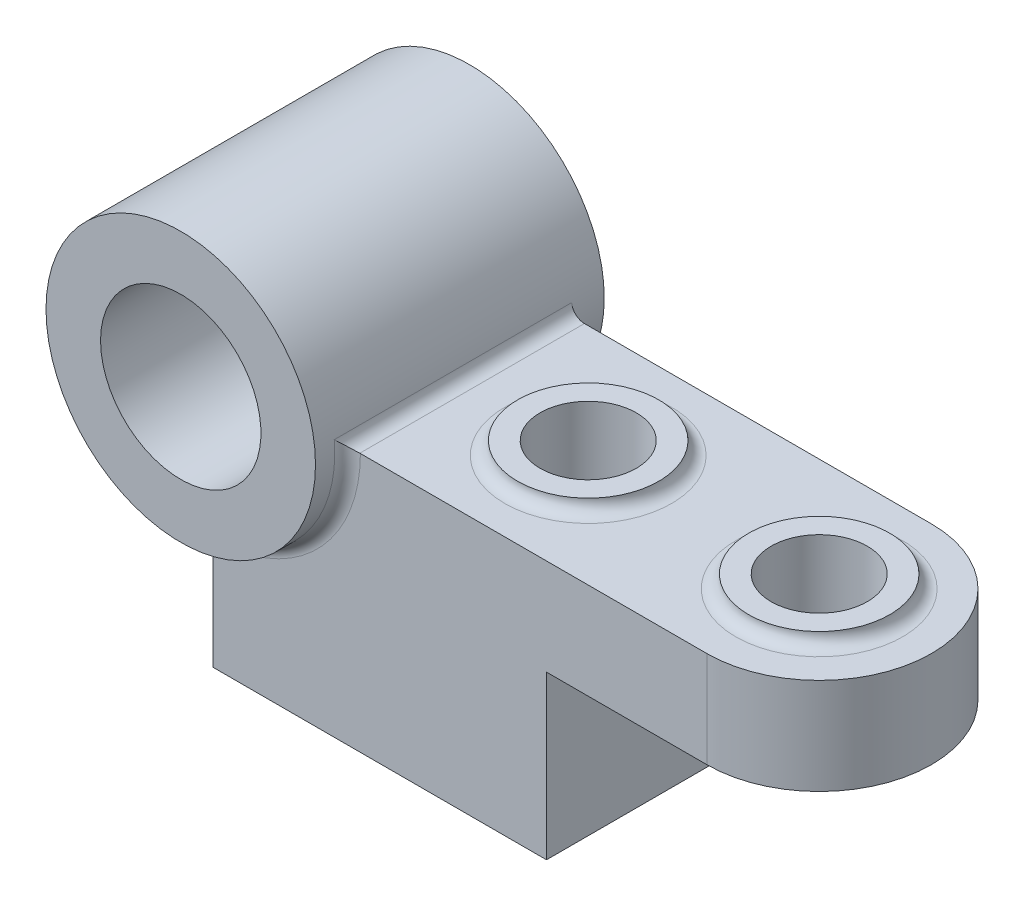
ISO-10303-21;
HEADER;
FILE_DESCRIPTION(('STEP AP214'),'2;1');
FILE_NAME('part.step','',(''),(''),'','','');
FILE_SCHEMA(('AUTOMOTIVE_DESIGN { 1 0 10303 214 1 1 1 1 }'));
ENDSEC;
DATA;
#1=APPLICATION_CONTEXT('core data for automotive mechanical design processes');
#2=APPLICATION_PROTOCOL_DEFINITION('international standard','automotive_design',2000,#1);
#3=PRODUCT_CONTEXT('',#1,'mechanical');
#4=PRODUCT('Part','Part','',(#3));
#5=PRODUCT_RELATED_PRODUCT_CATEGORY('part','',(#4));
#6=PRODUCT_DEFINITION_FORMATION('','',#4);
#7=PRODUCT_DEFINITION_CONTEXT('part definition',#1,'design');
#8=PRODUCT_DEFINITION('design','',#6,#7);
#9=PRODUCT_DEFINITION_SHAPE('','',#8);
#10=(LENGTH_UNIT() NAMED_UNIT(*) SI_UNIT(.MILLI.,.METRE.));
#11=(NAMED_UNIT(*) PLANE_ANGLE_UNIT() SI_UNIT($,.RADIAN.));
#12=(NAMED_UNIT(*) SI_UNIT($,.STERADIAN.) SOLID_ANGLE_UNIT());
#13=UNCERTAINTY_MEASURE_WITH_UNIT(LENGTH_MEASURE(1.E-05),#10,'distance_accuracy_value','');
#14=(GEOMETRIC_REPRESENTATION_CONTEXT(3) GLOBAL_UNCERTAINTY_ASSIGNED_CONTEXT((#13)) GLOBAL_UNIT_ASSIGNED_CONTEXT((#10,
#11,#12)) REPRESENTATION_CONTEXT('',''));
#15=CARTESIAN_POINT('',(0.,0.,0.));
#16=DIRECTION('',(0.,0.,1.));
#17=DIRECTION('',(1.,0.,0.));
#18=AXIS2_PLACEMENT_3D('',#15,#16,#17);
#19=CARTESIAN_POINT('',(0.,-15.,17.5));
#20=DIRECTION('',(0.,-1.,0.));
#21=DIRECTION('',(0.,0.,-1.));
#22=AXIS2_PLACEMENT_3D('',#19,#20,#21);
#23=PLANE('',#22);
#24=CARTESIAN_POINT('',(77.,-15.,0.));
#25=DIRECTION('',(0.,-1.,0.));
#26=DIRECTION('',(0.,0.,-1.));
#27=AXIS2_PLACEMENT_3D('',#24,#25,#26);
#28=CIRCLE('',#27,17.5);
#29=CARTESIAN_POINT('',(77.,-15.,17.5));
#30=VERTEX_POINT('',#29);
#31=CARTESIAN_POINT('',(77.,-15.,-17.5));
#32=VERTEX_POINT('',#31);
#33=EDGE_CURVE('E153',#30,#32,#28,.F.);
#34=ORIENTED_EDGE('',*,*,#33,.F.);
#35=DIRECTION('',(-1.,0.,0.));
#36=VECTOR('',#35,1.);
#37=CARTESIAN_POINT('',(0.,-15.,17.5));
#38=LINE('',#37,#36);
#39=CARTESIAN_POINT('',(52.,-15.,17.5));
#40=VERTEX_POINT('',#39);
#41=EDGE_CURVE('E180',#30,#40,#38,.T.);
#42=ORIENTED_EDGE('',*,*,#41,.T.);
#43=DIRECTION('',(0.,0.,-1.));
#44=VECTOR('',#43,1.);
#45=CARTESIAN_POINT('',(52.,-15.,17.5));
#46=LINE('',#45,#44);
#47=CARTESIAN_POINT('',(52.,-15.,-17.5));
#48=VERTEX_POINT('',#47);
#49=EDGE_CURVE('E182',#40,#48,#46,.T.);
#50=ORIENTED_EDGE('',*,*,#49,.T.);
#51=DIRECTION('',(-1.,0.,0.));
#52=VECTOR('',#51,1.);
#53=CARTESIAN_POINT('',(0.,-15.,-17.5));
#54=LINE('',#53,#52);
#55=EDGE_CURVE('E144',#32,#48,#54,.T.);
#56=ORIENTED_EDGE('',*,*,#55,.F.);
#57=EDGE_LOOP('',(#34,#42,#50,#56));
#58=FACE_BOUND('',#57,.T.);
#59=CARTESIAN_POINT('',(77.,-15.,0.));
#60=DIRECTION('',(0.,-1.,0.));
#61=DIRECTION('',(0.,0.,-1.));
#62=AXIS2_PLACEMENT_3D('',#59,#60,#61);
#63=CIRCLE('',#62,7.50000000000001);
#64=CARTESIAN_POINT('',(77.,-15.,-7.50000000000001));
#65=VERTEX_POINT('',#64);
#66=EDGE_CURVE('E169',#65,#65,#63,.T.);
#67=ORIENTED_EDGE('',*,*,#66,.F.);
#68=EDGE_LOOP('',(#67));
#69=FACE_BOUND('',#68,.T.);
#70=ADVANCED_FACE('F58',(#58,#69),#23,.T.);
#71=CARTESIAN_POINT('',(0.,0.,17.5));
#72=DIRECTION('',(0.,1.,0.));
#73=DIRECTION('',(0.,0.,1.));
#74=AXIS2_PLACEMENT_3D('',#71,#72,#73);
#75=PLANE('',#74);
#76=CARTESIAN_POINT('',(77.,0.,0.));
#77=DIRECTION('',(0.,1.,0.));
#78=DIRECTION('',(0.,0.,1.));
#79=AXIS2_PLACEMENT_3D('',#76,#77,#78);
#80=CIRCLE('',#79,13.);
#81=CARTESIAN_POINT('',(77.,0.,13.));
#82=VERTEX_POINT('',#81);
#83=EDGE_CURVE('E220',#82,#82,#80,.F.);
#84=ORIENTED_EDGE('',*,*,#83,.T.);
#85=EDGE_LOOP('',(#84));
#86=FACE_BOUND('',#85,.T.);
#87=CARTESIAN_POINT('',(41.,0.,0.));
#88=DIRECTION('',(0.,1.,0.));
#89=DIRECTION('',(0.,0.,1.));
#90=AXIS2_PLACEMENT_3D('',#87,#88,#89);
#91=CIRCLE('',#90,13.);
#92=CARTESIAN_POINT('',(41.,0.,13.));
#93=VERTEX_POINT('',#92);
#94=EDGE_CURVE('E212',#93,#93,#91,.F.);
#95=ORIENTED_EDGE('',*,*,#94,.T.);
#96=EDGE_LOOP('',(#95));
#97=FACE_BOUND('',#96,.T.);
#98=DIRECTION('',(1.,0.,0.));
#99=VECTOR('',#98,1.);
#100=CARTESIAN_POINT('',(0.,0.,-17.5));
#101=LINE('',#100,#99);
#102=CARTESIAN_POINT('',(22.9128784747792,0.,-17.5));
#103=VERTEX_POINT('',#102);
#104=CARTESIAN_POINT('',(77.,0.,-17.5));
#105=VERTEX_POINT('',#104);
#106=EDGE_CURVE('E139',#103,#105,#101,.T.);
#107=ORIENTED_EDGE('',*,*,#106,.F.);
#108=DIRECTION('',(0.,0.,-1.));
#109=VECTOR('',#108,1.);
#110=CARTESIAN_POINT('',(22.9128784747792,0.,17.5));
#111=LINE('',#110,#109);
#112=CARTESIAN_POINT('',(22.9128784747792,0.,17.5018984410588));
#113=VERTEX_POINT('',#112);
#114=EDGE_CURVE('E82',#103,#113,#111,.F.);
#115=ORIENTED_EDGE('',*,*,#114,.T.);
#116=CARTESIAN_POINT('',(23.,0.,19.5));
#117=DIRECTION('',(0.,1.,0.));
#118=DIRECTION('',(0.,0.,1.));
#119=AXIS2_PLACEMENT_3D('',#116,#117,#118);
#120=CIRCLE('',#119,2.);
#121=CARTESIAN_POINT('',(23.,0.,17.5));
#122=VERTEX_POINT('',#121);
#123=EDGE_CURVE('E230',#113,#122,#120,.F.);
#124=ORIENTED_EDGE('',*,*,#123,.T.);
#125=DIRECTION('',(1.,0.,0.));
#126=VECTOR('',#125,1.);
#127=CARTESIAN_POINT('',(0.,0.,17.5));
#128=LINE('',#127,#126);
#129=CARTESIAN_POINT('',(77.,0.,17.5));
#130=VERTEX_POINT('',#129);
#131=EDGE_CURVE('E160',#122,#130,#128,.T.);
#132=ORIENTED_EDGE('',*,*,#131,.T.);
#133=CARTESIAN_POINT('',(77.,0.,0.));
#134=DIRECTION('',(0.,1.,0.));
#135=DIRECTION('',(0.,0.,1.));
#136=AXIS2_PLACEMENT_3D('',#133,#134,#135);
#137=CIRCLE('',#136,17.5);
#138=EDGE_CURVE('E147',#105,#130,#137,.F.);
#139=ORIENTED_EDGE('',*,*,#138,.F.);
#140=EDGE_LOOP('',(#107,#115,#124,#132,#139));
#141=FACE_BOUND('',#140,.T.);
#142=ADVANCED_FACE('F156',(#86,#97,#141),#75,.T.);
#143=CARTESIAN_POINT('',(0.,0.,22.5));
#144=DIRECTION('',(0.,0.,-1.));
#145=DIRECTION('',(-1.,0.,0.));
#146=AXIS2_PLACEMENT_3D('',#143,#144,#145);
#147=CYLINDRICAL_SURFACE('',#146,12.5);
#148=CARTESIAN_POINT('',(0.,0.,22.5));
#149=DIRECTION('',(0.,0.,1.));
#150=DIRECTION('',(1.,0.,0.));
#151=AXIS2_PLACEMENT_3D('',#148,#149,#150);
#152=CIRCLE('',#151,12.5);
#153=CARTESIAN_POINT('',(-12.5,0.,22.5));
#154=VERTEX_POINT('',#153);
#155=EDGE_CURVE('E201',#154,#154,#152,.T.);
#156=CARTESIAN_POINT('',(0.,0.,-22.5));
#157=DIRECTION('',(0.,0.,1.));
#158=DIRECTION('',(1.,0.,0.));
#159=AXIS2_PLACEMENT_3D('',#156,#157,#158);
#160=CIRCLE('',#159,12.5);
#161=CARTESIAN_POINT('',(-12.5,0.,-22.5));
#162=VERTEX_POINT('',#161);
#163=EDGE_CURVE('E205',#162,#162,#160,.T.);
#164=CARTESIAN_POINT('',(-12.5,0.,22.5));
#165=CARTESIAN_POINT('',(-12.5,0.,22.03125));
#166=CARTESIAN_POINT('',(-12.5,0.,21.5625));
#167=CARTESIAN_POINT('',(-12.5,0.,20.625));
#168=CARTESIAN_POINT('',(-12.5,0.,20.15625));
#169=CARTESIAN_POINT('',(-12.5,0.,19.21875));
#170=CARTESIAN_POINT('',(-12.5,0.,18.75));
#171=CARTESIAN_POINT('',(-12.5,0.,17.8125));
#172=CARTESIAN_POINT('',(-12.5,0.,17.34375));
#173=CARTESIAN_POINT('',(-12.5,0.,16.40625));
#174=CARTESIAN_POINT('',(-12.5,0.,15.9375));
#175=CARTESIAN_POINT('',(-12.5,0.,15.));
#176=CARTESIAN_POINT('',(-12.5,0.,14.53125));
#177=CARTESIAN_POINT('',(-12.5,0.,13.59375));
#178=CARTESIAN_POINT('',(-12.5,0.,13.125));
#179=CARTESIAN_POINT('',(-12.5,0.,12.1875));
#180=CARTESIAN_POINT('',(-12.5,0.,11.71875));
#181=CARTESIAN_POINT('',(-12.5,0.,10.78125));
#182=CARTESIAN_POINT('',(-12.5,0.,10.3125));
#183=CARTESIAN_POINT('',(-12.5,0.,9.37499999999999));
#184=CARTESIAN_POINT('',(-12.5,0.,8.90625));
#185=CARTESIAN_POINT('',(-12.5,0.,7.96874999999999));
#186=CARTESIAN_POINT('',(-12.5,0.,7.5));
#187=CARTESIAN_POINT('',(-12.5,0.,6.5625));
#188=CARTESIAN_POINT('',(-12.5,0.,6.09374999999999));
#189=CARTESIAN_POINT('',(-12.5,0.,5.15624999999999));
#190=CARTESIAN_POINT('',(-12.5,0.,4.68749999999999));
#191=CARTESIAN_POINT('',(-12.5,0.,3.74999999999999));
#192=CARTESIAN_POINT('',(-12.5,0.,3.28124999999999));
#193=CARTESIAN_POINT('',(-12.5,0.,2.34375));
#194=CARTESIAN_POINT('',(-12.5,0.,1.87499999999999));
#195=CARTESIAN_POINT('',(-12.5,0.,0.937499999999994));
#196=CARTESIAN_POINT('',(-12.5,0.,0.468749999999993));
#197=CARTESIAN_POINT('',(-12.5,0.,-0.468750000000007));
#198=CARTESIAN_POINT('',(-12.5,0.,-0.937500000000008));
#199=CARTESIAN_POINT('',(-12.5,0.,-1.87500000000001));
#200=CARTESIAN_POINT('',(-12.5,0.,-2.34375000000001));
#201=CARTESIAN_POINT('',(-12.5,0.,-3.28125000000001));
#202=CARTESIAN_POINT('',(-12.5,0.,-3.75000000000001));
#203=CARTESIAN_POINT('',(-12.5,0.,-4.68750000000001));
#204=CARTESIAN_POINT('',(-12.5,0.,-5.15625000000001));
#205=CARTESIAN_POINT('',(-12.5,0.,-6.09375000000001));
#206=CARTESIAN_POINT('',(-12.5,0.,-6.56250000000001));
#207=CARTESIAN_POINT('',(-12.5,0.,-7.50000000000001));
#208=CARTESIAN_POINT('',(-12.5,0.,-7.96875000000001));
#209=CARTESIAN_POINT('',(-12.5,0.,-8.90625000000001));
#210=CARTESIAN_POINT('',(-12.5,0.,-9.37500000000001));
#211=CARTESIAN_POINT('',(-12.5,0.,-10.3125));
#212=CARTESIAN_POINT('',(-12.5,0.,-10.78125));
#213=CARTESIAN_POINT('',(-12.5,0.,-11.71875));
#214=CARTESIAN_POINT('',(-12.5,0.,-12.1875));
#215=CARTESIAN_POINT('',(-12.5,0.,-13.125));
#216=CARTESIAN_POINT('',(-12.5,0.,-13.59375));
#217=CARTESIAN_POINT('',(-12.5,0.,-14.53125));
#218=CARTESIAN_POINT('',(-12.5,0.,-15.));
#219=CARTESIAN_POINT('',(-12.5,0.,-15.9375));
#220=CARTESIAN_POINT('',(-12.5,0.,-16.40625));
#221=CARTESIAN_POINT('',(-12.5,0.,-17.34375));
#222=CARTESIAN_POINT('',(-12.5,0.,-17.8125));
#223=CARTESIAN_POINT('',(-12.5,0.,-18.75));
#224=CARTESIAN_POINT('',(-12.5,0.,-19.21875));
#225=CARTESIAN_POINT('',(-12.5,0.,-20.15625));
#226=CARTESIAN_POINT('',(-12.5,0.,-20.625));
#227=CARTESIAN_POINT('',(-12.5,0.,-21.5625));
#228=CARTESIAN_POINT('',(-12.5,0.,-22.03125));
#229=CARTESIAN_POINT('',(-12.5,0.,-22.5));
#230=B_SPLINE_CURVE_WITH_KNOTS('',3,(#164,#165,#166,#167,#168,#169,#170,#171,#172,#173,#174,
#175,#176,#177,#178,#179,#180,#181,#182,#183,#184,#185,#186,#187,#188,#189,#190,#191,#192,#193,
#194,#195,#196,#197,#198,#199,#200,#201,#202,#203,#204,#205,#206,#207,#208,#209,#210,#211,#212,
#213,#214,#215,#216,#217,#218,#219,#220,#221,#222,#223,#224,#225,#226,#227,#228,#229),
.UNSPECIFIED.,.F.,.F.,(4,2,2,2,2,2,2,2,2,2,2,2,2,2,2,2,2,2,2,2,2,2,2,2,2,2,2,2,2,2,2,2,4),(0.,
1.40625,2.8125,4.21875,5.625,7.03125,8.4375,9.84375,11.25,12.65625,14.0625,15.46875,16.875,
18.28125,19.6875,21.09375,22.5,23.90625,25.3125,26.71875,28.125,29.53125,30.9375,32.34375,33.75,
35.15625,36.5625,37.96875,39.375,40.78125,42.1875,43.59375,45.),.UNSPECIFIED.);
#231=EDGE_CURVE('BSEAM440',#154,#162,#230,.T.);
#232=ORIENTED_EDGE('',*,*,#155,.T.);
#233=ORIENTED_EDGE('',*,*,#163,.F.);
#234=ORIENTED_EDGE('',*,*,#231,.T.);
#235=ORIENTED_EDGE('',*,*,#231,.F.);
#236=EDGE_LOOP('',(#232,#234,#233,#235));
#237=FACE_BOUND('',#236,.T.);
#238=ADVANCED_FACE('F440',(#237),#147,.F.);
#239=CARTESIAN_POINT('',(0.,0.,22.5));
#240=DIRECTION('',(0.,0.,-1.));
#241=DIRECTION('',(-1.,0.,0.));
#242=AXIS2_PLACEMENT_3D('',#239,#240,#241);
#243=CYLINDRICAL_SURFACE('',#242,21.);
#244=DIRECTION('',(0.,0.,-1.));
#245=VECTOR('',#244,1.);
#246=CARTESIAN_POINT('',(0.,-21.,17.5));
#247=LINE('',#246,#245);
#248=CARTESIAN_POINT('',(0.,-21.,19.5));
#249=VERTEX_POINT('',#248);
#250=CARTESIAN_POINT('',(0.,-21.,-17.5));
#251=VERTEX_POINT('',#250);
#252=EDGE_CURVE('E200',#249,#251,#247,.T.);
#253=ORIENTED_EDGE('',*,*,#252,.F.);
#254=CARTESIAN_POINT('',(0.,0.,19.5));
#255=DIRECTION('',(0.,0.,1.));
#256=DIRECTION('',(1.,0.,0.));
#257=AXIS2_PLACEMENT_3D('',#254,#255,#256);
#258=CIRCLE('',#257,21.);
#259=CARTESIAN_POINT('',(20.920454259581,1.82608695652174,19.5));
#260=VERTEX_POINT('',#259);
#261=EDGE_CURVE('E224',#249,#260,#258,.T.);
#262=ORIENTED_EDGE('',*,*,#261,.T.);
#263=DIRECTION('',(0.,0.,-1.));
#264=VECTOR('',#263,1.);
#265=CARTESIAN_POINT('',(20.920454259581,1.82608695652174,22.5));
#266=LINE('',#265,#264);
#267=CARTESIAN_POINT('',(20.920454259581,1.82608695652174,-17.5));
#268=VERTEX_POINT('',#267);
#269=EDGE_CURVE('E219',#260,#268,#266,.T.);
#270=ORIENTED_EDGE('',*,*,#269,.T.);
#271=CARTESIAN_POINT('',(0.,0.,-17.5));
#272=DIRECTION('',(0.,0.,1.));
#273=DIRECTION('',(1.,0.,0.));
#274=AXIS2_PLACEMENT_3D('',#271,#272,#273);
#275=CIRCLE('',#274,21.);
#276=EDGE_CURVE('E172',#251,#268,#275,.T.);
#277=ORIENTED_EDGE('',*,*,#276,.F.);
#278=EDGE_LOOP('',(#253,#262,#270,#277));
#279=FACE_BOUND('',#278,.T.);
#280=CARTESIAN_POINT('',(0.,0.,22.5));
#281=DIRECTION('',(0.,0.,1.));
#282=DIRECTION('',(1.,0.,0.));
#283=AXIS2_PLACEMENT_3D('',#280,#281,#282);
#284=CIRCLE('',#283,21.);
#285=CARTESIAN_POINT('',(21.,0.,22.5));
#286=VERTEX_POINT('',#285);
#287=EDGE_CURVE('E152',#286,#286,#284,.T.);
#288=ORIENTED_EDGE('',*,*,#287,.F.);
#289=EDGE_LOOP('',(#288));
#290=FACE_BOUND('',#289,.T.);
#291=CARTESIAN_POINT('',(0.,0.,-22.5));
#292=DIRECTION('',(0.,0.,1.));
#293=DIRECTION('',(1.,0.,0.));
#294=AXIS2_PLACEMENT_3D('',#291,#292,#293);
#295=CIRCLE('',#294,21.);
#296=CARTESIAN_POINT('',(21.,0.,-22.5));
#297=VERTEX_POINT('',#296);
#298=EDGE_CURVE('E206',#297,#297,#295,.T.);
#299=ORIENTED_EDGE('',*,*,#298,.T.);
#300=EDGE_LOOP('',(#299));
#301=FACE_BOUND('',#300,.T.);
#302=ADVANCED_FACE('F242',(#279,#290,#301),#243,.T.);
#303=CARTESIAN_POINT('',(0.,0.,22.5));
#304=DIRECTION('',(0.,0.,1.));
#305=DIRECTION('',(1.,0.,0.));
#306=AXIS2_PLACEMENT_3D('',#303,#304,#305);
#307=PLANE('',#306);
#308=ORIENTED_EDGE('',*,*,#155,.F.);
#309=EDGE_LOOP('',(#308));
#310=FACE_BOUND('',#309,.T.);
#311=ORIENTED_EDGE('',*,*,#287,.T.);
#312=EDGE_LOOP('',(#311));
#313=FACE_BOUND('',#312,.T.);
#314=ADVANCED_FACE('F416',(#310,#313),#307,.T.);
#315=CARTESIAN_POINT('',(0.,0.,-22.5));
#316=DIRECTION('',(0.,0.,1.));
#317=DIRECTION('',(1.,0.,0.));
#318=AXIS2_PLACEMENT_3D('',#315,#316,#317);
#319=PLANE('',#318);
#320=ORIENTED_EDGE('',*,*,#163,.T.);
#321=EDGE_LOOP('',(#320));
#322=FACE_BOUND('',#321,.T.);
#323=ORIENTED_EDGE('',*,*,#298,.F.);
#324=EDGE_LOOP('',(#323));
#325=FACE_BOUND('',#324,.T.);
#326=ADVANCED_FACE('F409',(#322,#325),#319,.F.);
#327=CARTESIAN_POINT('',(0.,0.,17.5));
#328=DIRECTION('',(1.,0.,0.));
#329=DIRECTION('',(0.,0.,-1.));
#330=AXIS2_PLACEMENT_3D('',#327,#328,#329);
#331=PLANE('',#330);
#332=DIRECTION('',(0.,-1.,0.));
#333=VECTOR('',#332,1.);
#334=CARTESIAN_POINT('',(0.,0.,-17.5));
#335=LINE('',#334,#333);
#336=CARTESIAN_POINT('',(0.,-40.3391307266729,-17.5));
#337=VERTEX_POINT('',#336);
#338=EDGE_CURVE('E181',#251,#337,#335,.T.);
#339=ORIENTED_EDGE('',*,*,#338,.T.);
#340=DIRECTION('',(0.,0.,-1.));
#341=VECTOR('',#340,1.);
#342=CARTESIAN_POINT('',(0.,-40.3391307266729,17.5));
#343=LINE('',#342,#341);
#344=CARTESIAN_POINT('',(0.,-40.3391307266729,17.5));
#345=VERTEX_POINT('',#344);
#346=EDGE_CURVE('E198',#345,#337,#343,.T.);
#347=ORIENTED_EDGE('',*,*,#346,.F.);
#348=DIRECTION('',(0.,-1.,0.));
#349=VECTOR('',#348,1.);
#350=CARTESIAN_POINT('',(0.,0.,17.5));
#351=LINE('',#350,#349);
#352=CARTESIAN_POINT('',(0.,-23.,17.5));
#353=VERTEX_POINT('',#352);
#354=EDGE_CURVE('E145',#353,#345,#351,.T.);
#355=ORIENTED_EDGE('',*,*,#354,.F.);
#356=CARTESIAN_POINT('',(0.,-23.,19.5));
#357=DIRECTION('',(1.,0.,0.));
#358=DIRECTION('',(0.,0.,-1.));
#359=AXIS2_PLACEMENT_3D('',#356,#357,#358);
#360=CIRCLE('',#359,2.);
#361=EDGE_CURVE('E74',#353,#249,#360,.T.);
#362=ORIENTED_EDGE('',*,*,#361,.T.);
#363=ORIENTED_EDGE('',*,*,#252,.T.);
#364=EDGE_LOOP('',(#339,#347,#355,#362,#363));
#365=FACE_BOUND('',#364,.T.);
#366=ADVANCED_FACE('F235',(#365),#331,.F.);
#367=CARTESIAN_POINT('',(0.,-40.3391307266729,17.5));
#368=DIRECTION('',(0.,1.,0.));
#369=DIRECTION('',(0.,0.,1.));
#370=AXIS2_PLACEMENT_3D('',#367,#368,#369);
#371=PLANE('',#370);
#372=DIRECTION('',(1.,0.,0.));
#373=VECTOR('',#372,1.);
#374=CARTESIAN_POINT('',(0.,-40.3391307266729,-17.5));
#375=LINE('',#374,#373);
#376=CARTESIAN_POINT('',(52.,-40.3391307266729,-17.5));
#377=VERTEX_POINT('',#376);
#378=EDGE_CURVE('E183',#337,#377,#375,.T.);
#379=ORIENTED_EDGE('',*,*,#378,.T.);
#380=DIRECTION('',(0.,0.,-1.));
#381=VECTOR('',#380,1.);
#382=CARTESIAN_POINT('',(52.,-40.3391307266729,17.5));
#383=LINE('',#382,#381);
#384=CARTESIAN_POINT('',(52.,-40.3391307266729,17.5));
#385=VERTEX_POINT('',#384);
#386=EDGE_CURVE('E191',#385,#377,#383,.T.);
#387=ORIENTED_EDGE('',*,*,#386,.F.);
#388=DIRECTION('',(1.,0.,0.));
#389=VECTOR('',#388,1.);
#390=CARTESIAN_POINT('',(0.,-40.3391307266729,17.5));
#391=LINE('',#390,#389);
#392=EDGE_CURVE('E173',#345,#385,#391,.T.);
#393=ORIENTED_EDGE('',*,*,#392,.F.);
#394=ORIENTED_EDGE('',*,*,#346,.T.);
#395=EDGE_LOOP('',(#379,#387,#393,#394));
#396=FACE_BOUND('',#395,.T.);
#397=ADVANCED_FACE('F247',(#396),#371,.F.);
#398=CARTESIAN_POINT('',(52.,0.,17.5));
#399=DIRECTION('',(1.,0.,0.));
#400=DIRECTION('',(0.,0.,-1.));
#401=AXIS2_PLACEMENT_3D('',#398,#399,#400);
#402=PLANE('',#401);
#403=DIRECTION('',(0.,-1.,0.));
#404=VECTOR('',#403,1.);
#405=CARTESIAN_POINT('',(52.,0.,-17.5));
#406=LINE('',#405,#404);
#407=EDGE_CURVE('E188',#48,#377,#406,.T.);
#408=ORIENTED_EDGE('',*,*,#407,.F.);
#409=ORIENTED_EDGE('',*,*,#49,.F.);
#410=DIRECTION('',(0.,-1.,0.));
#411=VECTOR('',#410,1.);
#412=CARTESIAN_POINT('',(52.,0.,17.5));
#413=LINE('',#412,#411);
#414=EDGE_CURVE('E171',#40,#385,#413,.T.);
#415=ORIENTED_EDGE('',*,*,#414,.T.);
#416=ORIENTED_EDGE('',*,*,#386,.T.);
#417=EDGE_LOOP('',(#408,#409,#415,#416));
#418=FACE_BOUND('',#417,.T.);
#419=ADVANCED_FACE('F255',(#418),#402,.T.);
#420=CARTESIAN_POINT('',(0.,0.,17.5));
#421=DIRECTION('',(0.,0.,1.));
#422=DIRECTION('',(1.,0.,0.));
#423=AXIS2_PLACEMENT_3D('',#420,#421,#422);
#424=PLANE('',#423);
#425=ORIENTED_EDGE('',*,*,#131,.F.);
#426=CARTESIAN_POINT('',(0.,0.,17.5));
#427=DIRECTION('',(0.,0.,1.));
#428=DIRECTION('',(1.,0.,0.));
#429=AXIS2_PLACEMENT_3D('',#426,#427,#428);
#430=CIRCLE('',#429,23.);
#431=EDGE_CURVE('E90',#122,#353,#430,.F.);
#432=ORIENTED_EDGE('',*,*,#431,.T.);
#433=ORIENTED_EDGE('',*,*,#354,.T.);
#434=ORIENTED_EDGE('',*,*,#392,.T.);
#435=ORIENTED_EDGE('',*,*,#414,.F.);
#436=ORIENTED_EDGE('',*,*,#41,.F.);
#437=DIRECTION('',(0.,1.,0.));
#438=VECTOR('',#437,1.);
#439=CARTESIAN_POINT('',(77.,-25.,17.5));
#440=LINE('',#439,#438);
#441=EDGE_CURVE('E158',#30,#130,#440,.T.);
#442=ORIENTED_EDGE('',*,*,#441,.T.);
#443=EDGE_LOOP('',(#425,#432,#433,#434,#435,#436,#442));
#444=FACE_BOUND('',#443,.T.);
#445=ADVANCED_FACE('F246',(#444),#424,.T.);
#446=CARTESIAN_POINT('',(0.,0.,-17.5));
#447=DIRECTION('',(0.,0.,1.));
#448=DIRECTION('',(1.,0.,0.));
#449=AXIS2_PLACEMENT_3D('',#446,#447,#448);
#450=PLANE('',#449);
#451=ORIENTED_EDGE('',*,*,#276,.T.);
#452=CARTESIAN_POINT('',(22.9128784747792,2.,-17.5));
#453=DIRECTION('',(0.,0.,1.));
#454=DIRECTION('',(1.,0.,0.));
#455=AXIS2_PLACEMENT_3D('',#452,#453,#454);
#456=CIRCLE('',#455,2.);
#457=EDGE_CURVE('E12',#268,#103,#456,.T.);
#458=ORIENTED_EDGE('',*,*,#457,.T.);
#459=ORIENTED_EDGE('',*,*,#106,.T.);
#460=DIRECTION('',(0.,1.,0.));
#461=VECTOR('',#460,1.);
#462=CARTESIAN_POINT('',(77.,-25.,-17.5));
#463=LINE('',#462,#461);
#464=EDGE_CURVE('E138',#105,#32,#463,.F.);
#465=ORIENTED_EDGE('',*,*,#464,.T.);
#466=ORIENTED_EDGE('',*,*,#55,.T.);
#467=ORIENTED_EDGE('',*,*,#407,.T.);
#468=ORIENTED_EDGE('',*,*,#378,.F.);
#469=ORIENTED_EDGE('',*,*,#338,.F.);
#470=EDGE_LOOP('',(#451,#458,#459,#465,#466,#467,#468,#469));
#471=FACE_BOUND('',#470,.T.);
#472=ADVANCED_FACE('F136',(#471),#450,.F.);
#473=CARTESIAN_POINT('',(77.,-25.,0.));
#474=DIRECTION('',(0.,1.,0.));
#475=DIRECTION('',(0.,0.,1.));
#476=AXIS2_PLACEMENT_3D('',#473,#474,#475);
#477=CYLINDRICAL_SURFACE('',#476,17.5);
#478=ORIENTED_EDGE('',*,*,#33,.T.);
#479=ORIENTED_EDGE('',*,*,#464,.F.);
#480=ORIENTED_EDGE('',*,*,#138,.T.);
#481=ORIENTED_EDGE('',*,*,#441,.F.);
#482=EDGE_LOOP('',(#478,#479,#480,#481));
#483=FACE_BOUND('',#482,.T.);
#484=ADVANCED_FACE('F149',(#483),#477,.T.);
#485=CARTESIAN_POINT('',(77.,-25.,0.));
#486=DIRECTION('',(0.,1.,0.));
#487=DIRECTION('',(0.,0.,1.));
#488=AXIS2_PLACEMENT_3D('',#485,#486,#487);
#489=CYLINDRICAL_SURFACE('',#488,7.50000000000001);
#490=ORIENTED_EDGE('',*,*,#66,.T.);
#491=EDGE_LOOP('',(#490));
#492=FACE_BOUND('',#491,.T.);
#493=CARTESIAN_POINT('',(77.,2.,0.));
#494=DIRECTION('',(0.,1.,0.));
#495=DIRECTION('',(0.,0.,1.));
#496=AXIS2_PLACEMENT_3D('',#493,#494,#495);
#497=CIRCLE('',#496,7.50000000000001);
#498=CARTESIAN_POINT('',(77.,2.,7.50000000000001));
#499=VERTEX_POINT('',#498);
#500=EDGE_CURVE('E268',#499,#499,#497,.T.);
#501=ORIENTED_EDGE('',*,*,#500,.T.);
#502=EDGE_LOOP('',(#501));
#503=FACE_BOUND('',#502,.T.);
#504=ADVANCED_FACE('F261',(#492,#503),#489,.F.);
#505=CARTESIAN_POINT('',(0.,2.,0.));
#506=DIRECTION('',(0.,1.,0.));
#507=DIRECTION('',(0.,0.,1.));
#508=AXIS2_PLACEMENT_3D('',#505,#506,#507);
#509=PLANE('',#508);
#510=CARTESIAN_POINT('',(41.,2.,0.));
#511=DIRECTION('',(0.,1.,0.));
#512=DIRECTION('',(0.,0.,1.));
#513=AXIS2_PLACEMENT_3D('',#510,#511,#512);
#514=CIRCLE('',#513,7.50000000000001);
#515=CARTESIAN_POINT('',(41.,2.,7.50000000000001));
#516=VERTEX_POINT('',#515);
#517=EDGE_CURVE('E272',#516,#516,#514,.T.);
#518=ORIENTED_EDGE('',*,*,#517,.F.);
#519=EDGE_LOOP('',(#518));
#520=FACE_BOUND('',#519,.T.);
#521=CARTESIAN_POINT('',(41.,2.,0.));
#522=DIRECTION('',(0.,1.,0.));
#523=DIRECTION('',(0.,0.,1.));
#524=AXIS2_PLACEMENT_3D('',#521,#522,#523);
#525=CIRCLE('',#524,11.);
#526=CARTESIAN_POINT('',(41.,2.,11.));
#527=VERTEX_POINT('',#526);
#528=EDGE_CURVE('E162',#527,#527,#525,.T.);
#529=ORIENTED_EDGE('',*,*,#528,.T.);
#530=EDGE_LOOP('',(#529));
#531=FACE_BOUND('',#530,.T.);
#532=ADVANCED_FACE('F262',(#520,#531),#509,.T.);
#533=CARTESIAN_POINT('',(0.,-25.,0.));
#534=DIRECTION('',(0.,1.,0.));
#535=DIRECTION('',(0.,0.,1.));
#536=AXIS2_PLACEMENT_3D('',#533,#534,#535);
#537=PLANE('',#536);
#538=CARTESIAN_POINT('',(41.,-25.,0.));
#539=DIRECTION('',(0.,1.,0.));
#540=DIRECTION('',(0.,0.,1.));
#541=AXIS2_PLACEMENT_3D('',#538,#539,#540);
#542=CIRCLE('',#541,7.50000000000001);
#543=CARTESIAN_POINT('',(41.,-25.,7.50000000000001));
#544=VERTEX_POINT('',#543);
#545=EDGE_CURVE('E157',#544,#544,#542,.T.);
#546=ORIENTED_EDGE('',*,*,#545,.T.);
#547=EDGE_LOOP('',(#546));
#548=FACE_BOUND('',#547,.T.);
#549=ADVANCED_FACE('F331',(#548),#537,.T.);
#550=CARTESIAN_POINT('',(41.,-25.,0.));
#551=DIRECTION('',(0.,1.,0.));
#552=DIRECTION('',(0.,0.,1.));
#553=AXIS2_PLACEMENT_3D('',#550,#551,#552);
#554=CYLINDRICAL_SURFACE('',#553,7.50000000000001);
#555=ORIENTED_EDGE('',*,*,#545,.F.);
#556=EDGE_LOOP('',(#555));
#557=FACE_BOUND('',#556,.T.);
#558=ORIENTED_EDGE('',*,*,#517,.T.);
#559=EDGE_LOOP('',(#558));
#560=FACE_BOUND('',#559,.T.);
#561=ADVANCED_FACE('F322',(#557,#560),#554,.F.);
#562=CARTESIAN_POINT('',(0.,2.,0.));
#563=DIRECTION('',(0.,1.,0.));
#564=DIRECTION('',(0.,0.,1.));
#565=AXIS2_PLACEMENT_3D('',#562,#563,#564);
#566=PLANE('',#565);
#567=ORIENTED_EDGE('',*,*,#500,.F.);
#568=EDGE_LOOP('',(#567));
#569=FACE_BOUND('',#568,.T.);
#570=CARTESIAN_POINT('',(77.,2.,0.));
#571=DIRECTION('',(0.,1.,0.));
#572=DIRECTION('',(0.,0.,1.));
#573=AXIS2_PLACEMENT_3D('',#570,#571,#572);
#574=CIRCLE('',#573,11.);
#575=CARTESIAN_POINT('',(77.,2.,11.));
#576=VERTEX_POINT('',#575);
#577=EDGE_CURVE('E269',#576,#576,#574,.T.);
#578=ORIENTED_EDGE('',*,*,#577,.T.);
#579=EDGE_LOOP('',(#578));
#580=FACE_BOUND('',#579,.T.);
#581=ADVANCED_FACE('F292',(#569,#580),#566,.T.);
#582=CARTESIAN_POINT('',(77.,2.,0.));
#583=DIRECTION('',(0.,1.,0.));
#584=DIRECTION('',(0.,0.,1.));
#585=AXIS2_PLACEMENT_3D('',#582,#583,#584);
#586=TOROIDAL_SURFACE('',#585,13.,2.);
#587=ORIENTED_EDGE('',*,*,#83,.F.);
#588=EDGE_LOOP('',(#587));
#589=FACE_BOUND('',#588,.T.);
#590=ORIENTED_EDGE('',*,*,#577,.F.);
#591=EDGE_LOOP('',(#590));
#592=FACE_BOUND('',#591,.T.);
#593=ADVANCED_FACE('F283',(#589,#592),#586,.F.);
#594=CARTESIAN_POINT('',(41.,2.,0.));
#595=DIRECTION('',(0.,1.,0.));
#596=DIRECTION('',(0.,0.,1.));
#597=AXIS2_PLACEMENT_3D('',#594,#595,#596);
#598=TOROIDAL_SURFACE('',#597,13.,2.);
#599=ORIENTED_EDGE('',*,*,#94,.F.);
#600=EDGE_LOOP('',(#599));
#601=FACE_BOUND('',#600,.T.);
#602=ORIENTED_EDGE('',*,*,#528,.F.);
#603=EDGE_LOOP('',(#602));
#604=FACE_BOUND('',#603,.T.);
#605=ADVANCED_FACE('F282',(#601,#604),#598,.F.);
#606=CARTESIAN_POINT('',(22.9128784747792,2.,22.5));
#607=DIRECTION('',(0.,0.,-1.));
#608=DIRECTION('',(-1.,0.,0.));
#609=AXIS2_PLACEMENT_3D('',#606,#607,#608);
#610=CYLINDRICAL_SURFACE('',#609,2.);
#611=ORIENTED_EDGE('',*,*,#457,.F.);
#612=ORIENTED_EDGE('',*,*,#269,.F.);
#613=CARTESIAN_POINT('',(22.9128784747792,0.,17.5018984410588));
#614=CARTESIAN_POINT('',(22.8673259513623,-1.14888892978168E-05,17.5038727773799));
#615=CARTESIAN_POINT('',(22.8218534934656,0.00155583241429702,17.507427541133));
#616=CARTESIAN_POINT('',(22.7314994695228,0.00773043538466288,17.5175872646191));
#617=CARTESIAN_POINT('',(22.6866174034926,0.0123349498190578,17.5241894461614));
#618=CARTESIAN_POINT('',(22.5981933071995,0.0244116796673043,17.5402641215153));
#619=CARTESIAN_POINT('',(22.5546428166536,0.0318575153474078,17.5497100476907));
#620=CARTESIAN_POINT('',(22.4687812847612,0.0494358100140223,17.5713154933721));
#621=CARTESIAN_POINT('',(22.4264704646545,0.0595687453539524,17.5834754939529));
#622=CARTESIAN_POINT('',(22.3021006216417,0.0936152540864589,17.6236381738674));
#623=CARTESIAN_POINT('',(22.222218242009,0.121232010027149,17.6553961347678));
#624=CARTESIAN_POINT('',(22.0696292759871,0.184566855227295,17.7271710013132));
#625=CARTESIAN_POINT('',(21.9969405507992,0.220304417433907,17.767207737581));
#626=CARTESIAN_POINT('',(21.8278134091097,0.315985182710921,17.873638427168));
#627=CARTESIAN_POINT('',(21.7357184259187,0.379523421345338,17.9437121385047));
#628=CARTESIAN_POINT('',(21.5677279875703,0.515971824219716,18.0934439796112));
#629=CARTESIAN_POINT('',(21.4918698529685,0.588902975263991,18.1731235456711));
#630=CARTESIAN_POINT('',(21.3261477685996,0.773784626021595,18.3744399946071));
#631=CARTESIAN_POINT('',(21.2441281662209,0.889101812949919,18.4994679962312));
#632=CARTESIAN_POINT('',(21.1421202900642,1.06773935332127,18.6922577506891));
#633=CARTESIAN_POINT('',(21.1116116991903,1.12825912386267,18.757428049318));
#634=CARTESIAN_POINT('',(21.0572753575442,1.25084526347703,18.8890945992742));
#635=CARTESIAN_POINT('',(21.0334483250774,1.31291179805547,18.9555909923417));
#636=CARTESIAN_POINT('',(20.9650374065043,1.52106742696882,19.1779467868577));
#637=CARTESIAN_POINT('',(20.9345594394036,1.66994288918566,19.3359250598686));
#638=CARTESIAN_POINT('',(20.9208156456802,1.82198347775558,19.4956889403084));
#639=CARTESIAN_POINT('',(20.9206333706124,1.82403511592498,19.4978445085668));
#640=CARTESIAN_POINT('',(20.920454259581,1.82608695652174,19.5));
#641=B_SPLINE_CURVE_WITH_KNOTS('',3,(#613,#614,#615,#616,#617,#618,#619,#620,#621,#622,#623,
#624,#625,#626,#627,#628,#629,#630,#631,#632,#633,#634,#635,#636,#637,#638,#639,#640),
.UNSPECIFIED.,.F.,.F.,(4,2,2,2,2,2,2,2,2,2,2,2,2,4),(0.,0.136714137396307,0.273303884222993,
0.408655183405155,0.544030492938077,0.813607095886082,1.08383707081098,1.47766383789205,
1.87238632341786,2.4356062700004,2.71748596413811,2.99939595032904,3.65335182062182,
3.66229609762537),.UNSPECIFIED.);
#642=EDGE_CURVE('E61',#113,#260,#641,.T.);
#643=ORIENTED_EDGE('',*,*,#642,.F.);
#644=ORIENTED_EDGE('',*,*,#114,.F.);
#645=EDGE_LOOP('',(#611,#612,#643,#644));
#646=FACE_BOUND('',#645,.T.);
#647=ADVANCED_FACE('F65',(#646),#610,.F.);
#648=CARTESIAN_POINT('',(0.,0.,19.5));
#649=DIRECTION('',(0.,0.,1.));
#650=DIRECTION('',(1.,0.,0.));
#651=AXIS2_PLACEMENT_3D('',#648,#649,#650);
#652=TOROIDAL_SURFACE('',#651,23.,2.);
#653=ORIENTED_EDGE('',*,*,#361,.F.);
#654=ORIENTED_EDGE('',*,*,#431,.F.);
#655=ORIENTED_EDGE('',*,*,#123,.F.);
#656=ORIENTED_EDGE('',*,*,#642,.T.);
#657=ORIENTED_EDGE('',*,*,#261,.F.);
#658=EDGE_LOOP('',(#653,#654,#655,#656,#657));
#659=FACE_BOUND('',#658,.T.);
#660=ADVANCED_FACE('F240',(#659),#652,.F.);
#661=CLOSED_SHELL('',(#70,#142,#238,#302,#314,#326,#366,#397,#419,#445,#472,#484,#504,#532,#549,
#561,#581,#593,#605,#647,#660));
#662=MANIFOLD_SOLID_BREP('B2',#661);
#663=ADVANCED_BREP_SHAPE_REPRESENTATION('',(#18,#662),#14);
#664=SHAPE_DEFINITION_REPRESENTATION(#9,#663);
ENDSEC;
END-ISO-10303-21;
